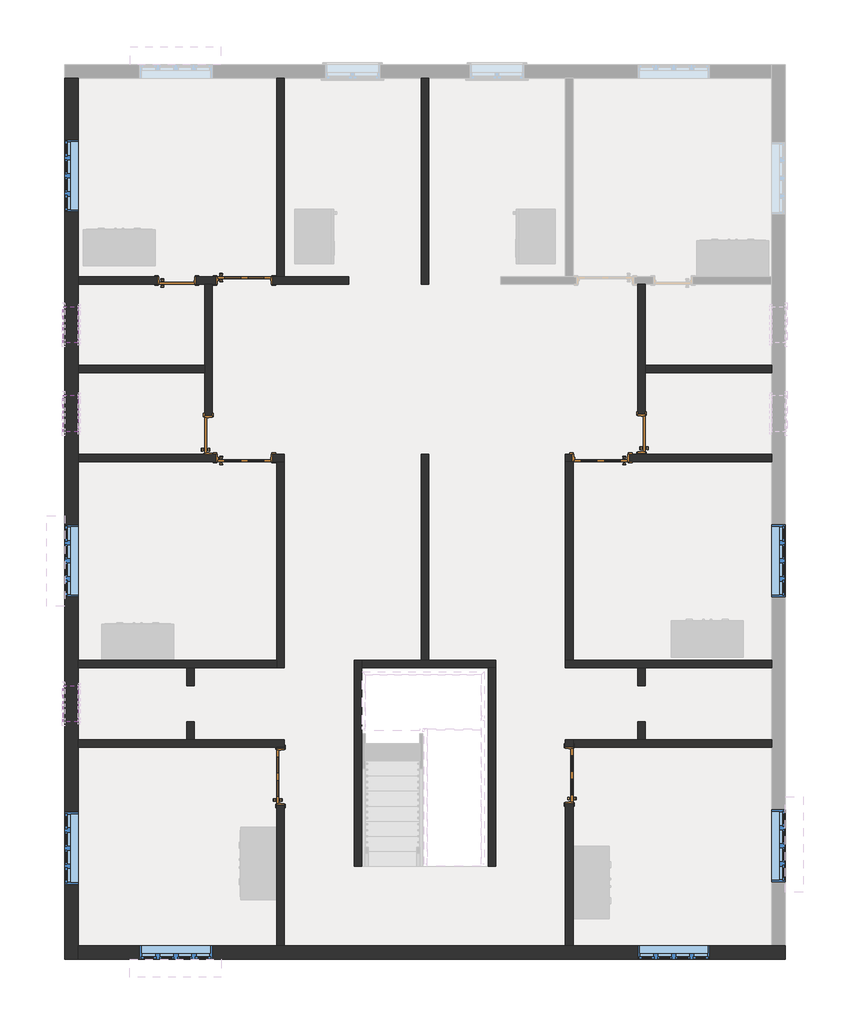
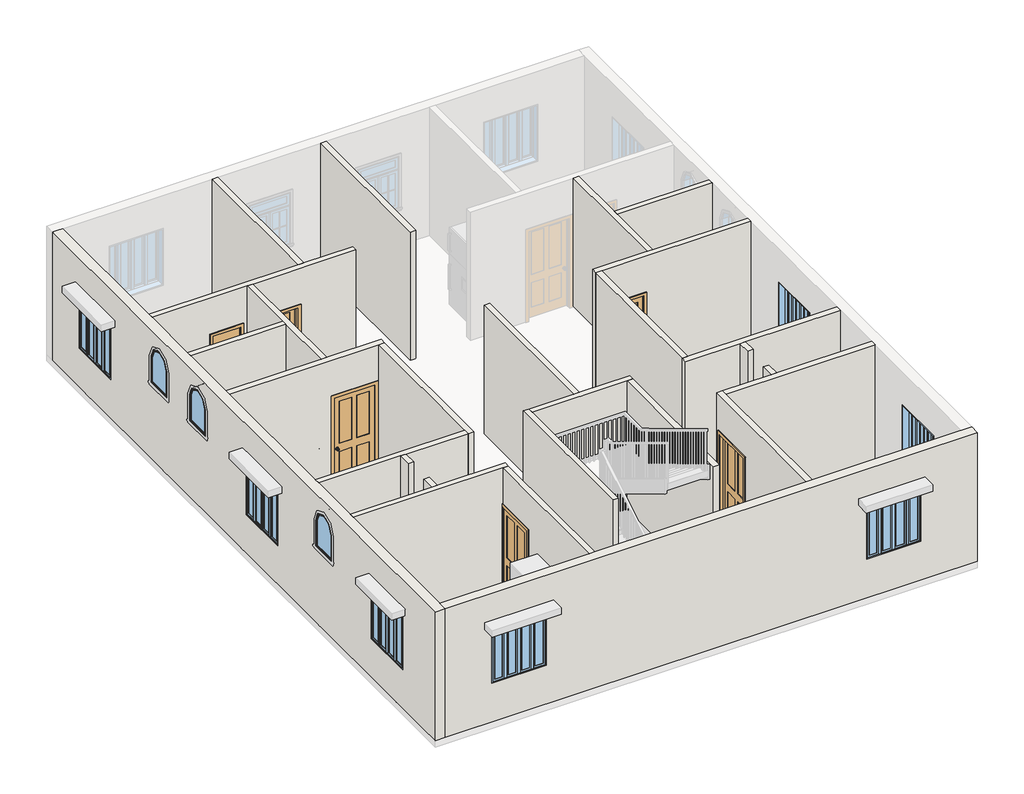
# One storey, part 1 of 4: 27 walls, 10 windows, 8 doors.
"""IFC4 building model written with IfcOpenShell, lengths in millimetres."""

from ifc_helpers import new_model, si_unit, frame, origin, place, context, project, spatial, polyline, circle_curve, outline, extrude, faceted_brep, transform, mapped, element, save
from ifc_brep_helpers import plane_surface, revolved_surface, advanced_brep
from components import door_a823658d, door_68a706ac, door_3f5f64ee, door_428b1ac9, window_casement_multi_sash_horizontal_main_windows_4_x_7_0e27d311, window_casement_multi_sash_horizontal_main_windows_4_x_7_c0e1ebbb, window_2fd4accf

model = new_model("IFC4")

# Units and contexts
model_context = context("Model", 3, world=origin())
ifc_project = project(units=[si_unit("LENGTHUNIT", "METRE", prefix="MILLI")], contexts=[model_context])

# Site, building, storey
site = spatial("IfcSite", under=ifc_project)
building = spatial("IfcBuilding", under=site)
storey = spatial("IfcBuildingStorey", under=building, Elevation=3352.8)

# Doors
placement = place(None, origin())
door_shape = door_a823658d(model_context)
element("IfcDoor", 1, ObjectType="Door-Interior-Single-4_Panel-Wood : 36\" x 84\"", at=placement, inside=storey, context=model_context, shape_type="MappedRepresentation", body=[
    mapped(door_shape, transform((-7097.4021954, -3420.7727897, 3352.8), x_axis=(0.0, 1.0, 0.0), y_axis=(-1.0, 0.0, 0.0), z_axis=(0.0, 0.0, 1.0))),
])
element("IfcDoor", 2, ObjectType="Door-Interior-Single-4_Panel-Wood : 36\" x 84\"", at=placement, inside=storey, context=model_context, shape_type="MappedRepresentation", body=[
    mapped(door_shape, transform((-12586.9771954, 1935.9816069, 3352.8), x_axis=(1.0, 0.0, 0.0), y_axis=(0.0, 1.0, 0.0), z_axis=(0.0, 0.0, 1.0))),
])
door_2_shape = door_68a706ac(model_context)
element("IfcDoor", 3, ObjectType="Door-Interior-Single-4_Panel-Wood : 36\" x 84\"", at=placement, inside=storey, context=model_context, shape_type="MappedRepresentation", body=[
    mapped(door_2_shape, transform((-11980.5521954, -3446.1727897, 3352.8), x_axis=(0.0, 1.0, 0.0), y_axis=(-1.0, 0.0, 0.0), z_axis=(0.0, 0.0, 1.0))),
])
element("IfcDoor", 4, ObjectType="Door-Interior-Single-4_Panel-Wood : 36\" x 84\"", at=placement, inside=storey, context=model_context, shape_type="MappedRepresentation", body=[
    mapped(door_2_shape, transform((-6567.1771954, 1935.9816069, 3352.8), x_axis=(-1.0, 0.0, 0.0), y_axis=(0.0, -1.0, 0.0), z_axis=(0.0, 0.0, 1.0))),
])
element("IfcDoor", 5, ObjectType="Door-Interior-Single-4_Panel-Wood : 36\" x 84\"", at=placement, inside=storey, context=model_context, shape_type="MappedRepresentation", body=[
    mapped(door_2_shape, transform((-12586.9771954, 4939.0022103, 3352.8), x_axis=(1.0, 0.0, 0.0), y_axis=(0.0, 1.0, 0.0), z_axis=(0.0, 0.0, 1.0))),
])
door_3_shape = door_3f5f64ee(model_context)
element("IfcDoor", 6, ObjectType="Door-Interior-Single-Flush_Panel-Wood : 24\" x 84\"", at=placement, inside=storey, context=model_context, shape_type="MappedRepresentation", body=[
    mapped(door_3_shape, transform((-13199.7521954, 2320.1566069, 3352.8), x_axis=(0.0, 1.0, 0.0), y_axis=(-1.0, 0.0, 0.0), z_axis=(0.0, 0.0, 1.0))),
])
door_4_shape = door_428b1ac9(model_context)
element("IfcDoor", 7, ObjectType="Door-Interior-Single-Flush_Panel-Wood : 24\" x 84\"", at=placement, inside=storey, context=model_context, shape_type="MappedRepresentation", body=[
    mapped(door_4_shape, transform((-13729.9771954, 4932.6522103, 3352.8), x_axis=(1.0, 0.0, 0.0), y_axis=(0.0, 1.0, 0.0), z_axis=(0.0, 0.0, 1.0))),
])
element("IfcDoor", 8, ObjectType="Door-Interior-Single-Flush_Panel-Wood : 24\" x 84\"", at=placement, inside=storey, context=model_context, shape_type="MappedRepresentation", body=[
    mapped(door_4_shape, transform((-5878.2021954, 2345.5566069, 3352.8), x_axis=(0.0, 1.0, 0.0), y_axis=(-1.0, 0.0, 0.0), z_axis=(0.0, 0.0, 1.0))),
])

# Walls
element("IfcWall", 9, ObjectType="INNER WALL 5\"", at=placement, inside=storey, context=model_context, shape_type="Brep", body=[
    faceted_brep([(-10821.6771954, 4872.3272103, 3352.8), (-10821.6771954, 4872.3272103, 6400.8), (-13133.0771954, 4872.3272103, 6400.8), (-13260.0771954, 4872.3272103, 6400.8), (-15395.2646954, 4872.3272103, 6400.8), (-15395.2646954, 4872.3272103, 3352.8), (-14060.1771954, 4872.3272103, 3352.8), (-14060.1771954, 4872.3272103, 5511.8), (-13399.7771954, 4872.3272103, 5511.8), (-13399.7771954, 4872.3272103, 3352.8), (-13260.0771954, 4872.3272103, 3352.8), (-13133.0771954, 4872.3272103, 3352.8), (-13069.5771954, 4872.3272103, 3352.8), (-13069.5771954, 4872.3272103, 5511.8), (-12104.3771954, 4872.3272103, 5511.8), (-12104.3771954, 4872.3272103, 3352.8), (-10821.6771954, 4999.3272103, 6400.8), (-10821.6771954, 4999.3272103, 3352.8), (-11913.8771954, 4999.3272103, 3352.8), (-12040.8771954, 4999.3272103, 3352.8), (-12104.3771954, 4999.3272103, 3352.8), (-12104.3771954, 4999.3272103, 5511.8), (-13069.5771954, 4999.3272103, 5511.8), (-13069.5771954, 4999.3272103, 3352.8), (-13399.7771954, 4999.3272103, 3352.8), (-13399.7771954, 4999.3272103, 5511.8), (-14060.1771954, 4999.3272103, 5511.8), (-14060.1771954, 4999.3272103, 3352.8), (-15395.2646954, 4999.3272103, 3352.8), (-15395.2646954, 4999.3272103, 6400.8), (-12040.8771954, 4999.3272103, 6400.8), (-11913.8771954, 4999.3272103, 6400.8)], [[[0, 1, 2, 3, 4, 5, 6, 7, 8, 9, 10, 11, 12, 13, 14, 15]], [[16, 17, 18, 19, 20, 21, 22, 23, 24, 25, 26, 27, 28, 29, 30, 31]], [[17, 0, 15, 20, 19, 18]], [[5, 28, 27, 6]], [[23, 12, 11, 10, 9, 24]], [[1, 0, 17, 16]], [[4, 3, 2, 1, 16, 31, 30, 29]], [[5, 4, 29, 28]], [[14, 21, 20, 15]], [[21, 14, 13, 22]], [[22, 13, 12, 23]], [[8, 25, 24, 9]], [[25, 8, 7, 26]], [[26, 7, 6, 27]]]),
])
element("IfcWall", 10, ObjectType="INNER WALL 5\"", at=placement, inside=storey, context=model_context, shape_type="SweptSolid", body=[
    extrude(outline(polyline([(-12040.8771954, 4999.3272103), (-12040.8771954, 8352.1272103), (-11913.8771954, 8352.1272103), (-11913.8771954, 4999.3272103), (-12040.8771954, 4999.3272103)])), frame((0.0, 0.0, 3352.8), z_axis=(0.0, 0.0, 1.0), x_axis=(1.0, 0.0, 0.0)), (0.0, 0.0, 1.0), 3048.0),
])
element("IfcWall", 11, ObjectType="INNER WALL 5\"", at=placement, inside=storey, context=model_context, shape_type="SweptSolid", body=[
    extrude(outline(polyline([(-9602.4771954, 4872.3272103), (-9602.4771954, 8352.1272103), (-9475.4771954, 8352.1272103), (-9475.4771954, 4872.3272103), (-9602.4771954, 4872.3272103)])), frame((0.0, 0.0, 3352.8), z_axis=(0.0, 0.0, 1.0), x_axis=(1.0, 0.0, 0.0)), (0.0, 0.0, 1.0), 3048.0),
])
element("IfcWall", 12, ObjectType="INNER WALL 5\"", at=placement, inside=storey, context=model_context, shape_type="SweptSolid", body=[
    extrude(outline(polyline([(-13260.0771954, 3373.7272103), (-15395.2646954, 3373.7272103), (-15395.2646954, 3500.7272103), (-13260.0771954, 3500.7272103), (-13260.0771954, 3373.7272103)])), frame((0.0, 0.0, 3352.8), z_axis=(0.0, 0.0, 1.0), x_axis=(1.0, 0.0, 0.0)), (0.0, 0.0, 1.0), 3048.0),
])
element("IfcWall", 13, ObjectType="INNER WALL 5\"", at=placement, inside=storey, context=model_context, shape_type="Brep", body=[
    faceted_brep([(-13260.0771954, 2002.6566069, 6400.8), (-13260.0771954, 3373.7272103, 6400.8), (-13260.0771954, 3500.7272103, 6400.8), (-13260.0771954, 4872.3272103, 6400.8), (-13260.0771954, 4872.3272103, 3352.8), (-13260.0771954, 3500.7272103, 3352.8), (-13260.0771954, 3373.7272103, 3352.8), (-13260.0771954, 2650.3566069, 3352.8), (-13260.0771954, 2650.3566069, 5511.8), (-13260.0771954, 2002.6566069, 5511.8), (-13133.0771954, 4872.3272103, 6400.8), (-13133.0771954, 2002.6566069, 6400.8), (-13133.0771954, 2002.6566069, 5511.8), (-13133.0771954, 2650.3566069, 5511.8), (-13133.0771954, 2650.3566069, 3352.8), (-13133.0771954, 4872.3272103, 3352.8)], [[[0, 1, 2, 3, 4, 5, 6, 7, 8, 9]], [[10, 11, 12, 13, 14, 15]], [[4, 15, 14, 7, 6, 5]], [[3, 2, 1, 0, 11, 10]], [[4, 3, 10, 15]], [[11, 0, 9, 12]], [[13, 8, 7, 14]], [[8, 13, 12, 9]]]),
])
element("IfcWall", 14, ObjectType="INNER WALL 5\"", at=placement, inside=storey, context=model_context, shape_type="Brep", body=[
    faceted_brep([(-11913.8771954, 1875.6566069, 6400.8), (-12040.8771954, 1875.6566069, 6400.8), (-15395.2646954, 1875.6566069, 6400.8), (-15395.2646954, 1875.6566069, 3352.8), (-13069.5771954, 1875.6566069, 3352.8), (-13069.5771954, 1875.6566069, 5511.8), (-12104.3771954, 1875.6566069, 5511.8), (-12104.3771954, 1875.6566069, 3352.8), (-12040.8771954, 1875.6566069, 3352.8), (-11913.8771954, 1875.6566069, 3352.8), (-15395.2646954, 2002.6566069, 6400.8), (-13260.0771954, 2002.6566069, 6400.8), (-13133.0771954, 2002.6566069, 6400.8), (-11913.8771954, 2002.6566069, 6400.8), (-11913.8771954, 2002.6566069, 3352.8), (-12104.3771954, 2002.6566069, 3352.8), (-12104.3771954, 2002.6566069, 5511.8), (-13069.5771954, 2002.6566069, 5511.8), (-13069.5771954, 2002.6566069, 3352.8), (-13133.0771954, 2002.6566069, 3352.8), (-13133.0771954, 2002.6566069, 5511.8), (-13260.0771954, 2002.6566069, 5511.8), (-13260.0771954, 2002.6566069, 3352.8), (-15395.2646954, 2002.6566069, 3352.8), (-13260.0771954, 1989.9566069, 3352.8), (-13133.0771954, 1989.9566069, 3352.8), (-13133.0771954, 1989.9566069, 5511.8), (-13260.0771954, 1989.9566069, 5511.8)], [[[0, 1, 2, 3, 4, 5, 6, 7, 8, 9]], [[10, 11, 12, 13, 14, 15, 16, 17, 18, 19, 20, 21, 22, 23]], [[3, 23, 22, 24, 25, 19, 18, 4]], [[14, 9, 8, 7, 15]], [[2, 1, 0, 13, 12, 11, 10]], [[3, 2, 10, 23]], [[0, 9, 14, 13]], [[6, 16, 15, 7]], [[16, 6, 5, 17]], [[17, 5, 4, 18]], [[25, 26, 20, 19]], [[27, 24, 22, 21]], [[26, 27, 21, 20]], [[26, 25, 24, 27]]]),
])
element("IfcWall", 15, ObjectType="INNER WALL 5\"", at=placement, inside=storey, context=model_context, shape_type="SweptSolid", body=[
    extrude(outline(polyline([(-9602.4771954, -1477.6727897), (-9602.4771954, 2002.6566069), (-9475.4771954, 2002.6566069), (-9475.4771954, -1477.6727897), (-9602.4771954, -1477.6727897)])), frame((0.0, 0.0, 3352.8), z_axis=(0.0, 0.0, 1.0), x_axis=(1.0, 0.0, 0.0)), (0.0, 0.0, 1.0), 3048.0),
])
element("IfcWall", 16, ObjectType="INNER WALL 5\"", at=placement, inside=storey, context=model_context, shape_type="Brep", body=[
    faceted_brep([(-5944.8771954, 2002.6566069, 6400.8), (-5944.8771954, 4872.3272103, 6400.8), (-5944.8771954, 4872.3272103, 3352.8), (-5944.8771954, 2675.7566069, 3352.8), (-5944.8771954, 2675.7566069, 5511.8), (-5944.8771954, 2015.3566069, 5511.8), (-5944.8771954, 2015.3566069, 3352.8), (-5944.8771954, 2002.6566069, 3352.8), (-5817.8771954, 4872.3272103, 6400.8), (-5817.8771954, 3500.7272103, 6400.8), (-5817.8771954, 3373.7272103, 6400.8), (-5817.8771954, 2002.6566069, 6400.8), (-5817.8771954, 2002.6566069, 3352.8), (-5817.8771954, 2015.3566069, 3352.8), (-5817.8771954, 2015.3566069, 5511.8), (-5817.8771954, 2675.7566069, 5511.8), (-5817.8771954, 2675.7566069, 3352.8), (-5817.8771954, 3373.7272103, 3352.8), (-5817.8771954, 3500.7272103, 3352.8), (-5817.8771954, 4872.3272103, 3352.8)], [[[0, 1, 2, 3, 4, 5, 6, 7]], [[8, 9, 10, 11, 12, 13, 14, 15, 16, 17, 18, 19]], [[2, 19, 18, 17, 16, 3]], [[12, 7, 6, 13]], [[1, 0, 11, 10, 9, 8]], [[2, 1, 8, 19]], [[0, 7, 12, 11]], [[15, 4, 3, 16]], [[4, 15, 14, 5]], [[5, 14, 13, 6]]]),
])
element("IfcWall", 17, ObjectType="INNER WALL 5\"", at=placement, inside=storey, context=model_context, shape_type="SweptSolid", body=[
    extrude(outline(polyline([(-3684.2771954, 3373.7272103), (-5817.8771954, 3373.7272103), (-5817.8771954, 3500.7272103), (-3684.2771954, 3500.7272103), (-3684.2771954, 3373.7272103)])), frame((0.0, 0.0, 3352.8), z_axis=(0.0, 0.0, 1.0), x_axis=(1.0, 0.0, 0.0)), (0.0, 0.0, 1.0), 3048.0),
])
element("IfcWall", 18, ObjectType="INNER WALL 5\"", at=placement, inside=storey, context=model_context, shape_type="Brep", body=[
    faceted_brep([(-7164.0771954, 2002.6566069, 6400.8), (-5944.8771954, 2002.6566069, 6400.8), (-5817.8771954, 2002.6566069, 6400.8), (-3684.2771954, 2002.6566069, 6400.8), (-3684.2771954, 2002.6566069, 3352.8), (-5817.8771954, 2002.6566069, 3352.8), (-5944.8771954, 2002.6566069, 3352.8), (-6084.5771954, 2002.6566069, 3352.8), (-6084.5771954, 2002.6566069, 5511.8), (-7049.7771954, 2002.6566069, 5511.8), (-7049.7771954, 2002.6566069, 3352.8), (-7164.0771954, 2002.6566069, 3352.8), (-3684.2771954, 1875.6566069, 6400.8), (-7037.0771954, 1875.6566069, 6400.8), (-7164.0771954, 1875.6566069, 6400.8), (-7164.0771954, 1875.6566069, 3352.8), (-7049.7771954, 1875.6566069, 3352.8), (-7049.7771954, 1875.6566069, 5511.8), (-6084.5771954, 1875.6566069, 5511.8), (-6084.5771954, 1875.6566069, 3352.8), (-3684.2771954, 1875.6566069, 3352.8)], [[[0, 1, 2, 3, 4, 5, 6, 7, 8, 9, 10, 11]], [[12, 13, 14, 15, 16, 17, 18, 19, 20]], [[4, 20, 19, 7, 6, 5]], [[15, 11, 10, 16]], [[3, 2, 1, 0, 14, 13, 12]], [[4, 3, 12, 20]], [[0, 11, 15, 14]], [[9, 17, 16, 10]], [[17, 9, 8, 18]], [[18, 8, 7, 19]]]),
])
element("IfcWall", 19, ObjectType="INNER WALL 5\"", at=placement, inside=storey, context=model_context, shape_type="Brep", body=[
    faceted_brep([(-12040.8771954, 1875.6566069, 3352.8), (-12040.8771954, -1477.6727897, 3352.8), (-12040.8771954, -1604.6727897, 3352.8), (-12040.8771954, -1604.6727897, 6400.8), (-12040.8771954, -1477.6727897, 6400.8), (-12040.8771954, 1875.6566069, 6400.8), (-11913.8771954, 1875.6566069, 3352.8), (-11913.8771954, 1875.6566069, 6400.8), (-11913.8771954, -1604.6727897, 6400.8), (-11913.8771954, -1604.6727897, 3352.8)], [[[0, 1, 2, 3, 4, 5]], [[6, 7, 8, 9]], [[2, 1, 0, 6, 9]], [[5, 4, 3, 8, 7]], [[0, 5, 7, 6]], [[3, 2, 9, 8]]]),
])
element("IfcWall", 20, ObjectType="INNER WALL 5\"", at=placement, inside=storey, context=model_context, shape_type="Brep", body=[
    faceted_brep([(-12040.8771954, -1477.6727897, 3352.8), (-15395.2646954, -1477.6727897, 3352.8), (-15395.2646954, -1477.6727897, 6400.8), (-12040.8771954, -1477.6727897, 6400.8), (-12040.8771954, -1604.6727897, 3352.8), (-12040.8771954, -1604.6727897, 6400.8), (-13437.8771954, -1604.6727897, 6400.8), (-13564.8771954, -1604.6727897, 6400.8), (-15395.2646954, -1604.6727897, 6400.8), (-15395.2646954, -1604.6727897, 3352.8), (-13564.8771954, -1604.6727897, 3352.8), (-13437.8771954, -1604.6727897, 3352.8)], [[[0, 1, 2, 3]], [[4, 5, 6, 7, 8, 9, 10, 11]], [[1, 0, 4, 11, 10, 9]], [[3, 2, 8, 7, 6, 5]], [[0, 3, 5, 4]], [[2, 1, 9, 8]]]),
])
element("IfcWall", 21, ObjectType="INNER WALL 5\"", at=placement, inside=storey, context=model_context, shape_type="Brep", body=[
    faceted_brep([(-15395.2646954, -2950.8727897, 3352.8), (-12040.8771954, -2950.8727897, 3352.8), (-11913.8771954, -2950.8727897, 3352.8), (-11913.8771954, -2950.8727897, 6400.8), (-12040.8771954, -2950.8727897, 6400.8), (-15395.2646954, -2950.8727897, 6400.8), (-15395.2646954, -2823.8727897, 3352.8), (-15395.2646954, -2823.8727897, 6400.8), (-13564.8771954, -2823.8727897, 6400.8), (-13437.8771954, -2823.8727897, 6400.8), (-11913.8771954, -2823.8727897, 6400.8), (-11913.8771954, -2823.8727897, 3352.8), (-13437.8771954, -2823.8727897, 3352.8), (-13564.8771954, -2823.8727897, 3352.8)], [[[0, 1, 2, 3, 4, 5]], [[6, 7, 8, 9, 10, 11, 12, 13]], [[2, 1, 0, 6, 13, 12, 11]], [[5, 4, 3, 10, 9, 8, 7]], [[0, 5, 7, 6]], [[3, 2, 11, 10]]]),
])
element("IfcWall", 22, ObjectType="INNER WALL 5\"", at=placement, inside=storey, context=model_context, shape_type="SweptSolid", body=[
    extrude(outline(polyline([(-6303.6727897, 6400.8), (-2950.8727897, 6400.8), (-2950.8727897, 3352.8), (-2963.5727897, 3352.8), (-2963.5727897, 5511.8), (-3928.7727897, 5511.8), (-3928.7727897, 3352.8), (-6303.6727897, 3352.8), (-6303.6727897, 6400.8)])), frame((-12040.8771954, 0.0, 0.0), z_axis=(1.0, 0.0, 0.0), x_axis=(0.0, 1.0, 0.0)), (0.0, 0.0, 1.0), 127.0),
])
element("IfcWall", 23, ObjectType="INNER WALL 5\"", at=placement, inside=storey, context=model_context, shape_type="Brep", body=[
    faceted_brep([(-7037.0771954, -2823.8727897, 6400.8), (-7037.0771954, -2950.8727897, 6400.8), (-7037.0771954, -6303.6727897, 6400.8), (-7037.0771954, -6303.6727897, 3352.8), (-7037.0771954, -3903.3727897, 3352.8), (-7037.0771954, -3903.3727897, 5511.8), (-7037.0771954, -2938.1727897, 5511.8), (-7037.0771954, -2938.1727897, 3352.8), (-7037.0771954, -2823.8727897, 3352.8), (-7164.0771954, -6303.6727897, 6400.8), (-7164.0771954, -2823.8727897, 6400.8), (-7164.0771954, -2823.8727897, 3352.8), (-7164.0771954, -2938.1727897, 3352.8), (-7164.0771954, -2938.1727897, 5511.8), (-7164.0771954, -3903.3727897, 5511.8), (-7164.0771954, -3903.3727897, 3352.8), (-7164.0771954, -6303.6727897, 3352.8)], [[[0, 1, 2, 3, 4, 5, 6, 7, 8]], [[9, 10, 11, 12, 13, 14, 15, 16]], [[3, 16, 15, 4]], [[11, 8, 7, 12]], [[2, 1, 0, 10, 9]], [[3, 2, 9, 16]], [[0, 8, 11, 10]], [[6, 13, 12, 7]], [[13, 6, 5, 14]], [[14, 5, 4, 15]]]),
])
element("IfcWall", 24, ObjectType="INNER WALL 5\"", at=placement, inside=storey, context=model_context, shape_type="Brep", body=[
    faceted_brep([(-3684.2771954, -2823.8727897, 3352.8), (-5817.8771954, -2823.8727897, 3352.8), (-5944.8771954, -2823.8727897, 3352.8), (-7037.0771954, -2823.8727897, 3352.8), (-7037.0771954, -2823.8727897, 6400.8), (-5944.8771954, -2823.8727897, 6400.8), (-5817.8771954, -2823.8727897, 6400.8), (-3684.2771954, -2823.8727897, 6400.8), (-3684.2771954, -2950.8727897, 3352.8), (-3684.2771954, -2950.8727897, 6400.8), (-7037.0771954, -2950.8727897, 6400.8), (-7037.0771954, -2950.8727897, 3352.8)], [[[0, 1, 2, 3, 4, 5, 6, 7]], [[8, 9, 10, 11]], [[3, 2, 1, 0, 8, 11]], [[7, 6, 5, 4, 10, 9]], [[4, 3, 11, 10]], [[0, 7, 9, 8]]]),
])
element("IfcWall", 25, ObjectType="INNER WALL 5\"", at=placement, inside=storey, context=model_context, shape_type="Brep", body=[
    faceted_brep([(-3684.2771954, -1477.6727897, 3352.8), (-7037.0771954, -1477.6727897, 3352.8), (-7164.0771954, -1477.6727897, 3352.8), (-7164.0771954, -1477.6727897, 6400.8), (-7037.0771954, -1477.6727897, 6400.8), (-3684.2771954, -1477.6727897, 6400.8), (-3684.2771954, -1604.6727897, 3352.8), (-3684.2771954, -1604.6727897, 6400.8), (-5817.8771954, -1604.6727897, 6400.8), (-5944.8771954, -1604.6727897, 6400.8), (-7164.0771954, -1604.6727897, 6400.8), (-7164.0771954, -1604.6727897, 3352.8), (-5944.8771954, -1604.6727897, 3352.8), (-5817.8771954, -1604.6727897, 3352.8)], [[[0, 1, 2, 3, 4, 5]], [[6, 7, 8, 9, 10, 11, 12, 13]], [[2, 1, 0, 6, 13, 12, 11]], [[5, 4, 3, 10, 9, 8, 7]], [[0, 5, 7, 6]], [[3, 2, 11, 10]]]),
])
element("IfcWall", 26, ObjectType="INNER WALL 5\"", at=placement, inside=storey, context=model_context, shape_type="SweptSolid", body=[
    extrude(outline(polyline([(-7037.0771954, 1875.6566069), (-7037.0771954, -1477.6727897), (-7164.0771954, -1477.6727897), (-7164.0771954, 1875.6566069), (-7037.0771954, 1875.6566069)])), frame((0.0, 0.0, 3352.8), z_axis=(0.0, 0.0, 1.0), x_axis=(1.0, 0.0, 0.0)), (0.0, 0.0, 1.0), 3048.0),
])
element("IfcWall", 27, ObjectType="INNER WALL 5\"", at=placement, inside=storey, context=model_context, shape_type="SweptSolid", body=[
    extrude(outline(polyline([(-13564.8771954, -1909.4727897), (-13564.8771954, -1604.6727897), (-13437.8771954, -1604.6727897), (-13437.8771954, -1909.4727897), (-13564.8771954, -1909.4727897)])), frame((0.0, 0.0, 3352.8), z_axis=(0.0, 0.0, 1.0), x_axis=(1.0, 0.0, 0.0)), (0.0, 0.0, 1.0), 3048.0),
])
element("IfcWall", 28, ObjectType="INNER WALL 5\"", at=placement, inside=storey, context=model_context, shape_type="SweptSolid", body=[
    extrude(outline(polyline([(-13437.8771954, -2519.0727897), (-13437.8771954, -2823.8727897), (-13564.8771954, -2823.8727897), (-13564.8771954, -2519.0727897), (-13437.8771954, -2519.0727897)])), frame((0.0, 0.0, 3352.8), z_axis=(0.0, 0.0, 1.0), x_axis=(1.0, 0.0, 0.0)), (0.0, 0.0, 1.0), 3048.0),
])
element("IfcWall", 29, ObjectType="INNER WALL 5\"", at=placement, inside=storey, context=model_context, shape_type="SweptSolid", body=[
    extrude(outline(polyline([(-5817.8771954, -2519.0727897), (-5817.8771954, -2823.8727897), (-5944.8771954, -2823.8727897), (-5944.8771954, -2519.0727897), (-5817.8771954, -2519.0727897)])), frame((0.0, 0.0, 3352.8), z_axis=(0.0, 0.0, 1.0), x_axis=(1.0, 0.0, 0.0)), (0.0, 0.0, 1.0), 3048.0),
])
element("IfcWall", 30, ObjectType="INNER WALL 5\"", at=placement, inside=storey, context=model_context, shape_type="SweptSolid", body=[
    extrude(outline(polyline([(-5944.8771954, -1909.4727897), (-5944.8771954, -1604.6727897), (-5817.8771954, -1604.6727897), (-5817.8771954, -1909.4727897), (-5944.8771954, -1909.4727897)])), frame((0.0, 0.0, 3352.8), z_axis=(0.0, 0.0, 1.0), x_axis=(1.0, 0.0, 0.0)), (0.0, 0.0, 1.0), 3048.0),
])
element("IfcWall", 31, ObjectType="INNER WALL 5\"", at=placement, inside=storey, context=model_context, shape_type="Brep", body=[
    faceted_brep([(-10605.7771954, -4957.4727897, 3352.8), (-10605.7771954, -1604.6727897, 3352.8), (-10605.7771954, -1477.6727897, 3352.8), (-10605.7771954, -1477.6727897, 6400.8), (-10605.7771954, -1604.6727897, 6400.8), (-10605.7771954, -4957.4727897, 6400.8), (-10732.7771954, -4957.4727897, 3352.8), (-10732.7771954, -4957.4727897, 6400.8), (-10732.7771954, -1477.6727897, 6400.8), (-10732.7771954, -1477.6727897, 3352.8)], [[[0, 1, 2, 3, 4, 5]], [[6, 7, 8, 9]], [[2, 1, 0, 6, 9]], [[5, 4, 3, 8, 7]], [[0, 5, 7, 6]], [[3, 2, 9, 8]]]),
])
element("IfcWall", 32, ObjectType="INNER WALL 5\"", at=placement, inside=storey, context=model_context, shape_type="Brep", body=[
    faceted_brep([(-10605.7771954, -1604.6727897, 3352.8), (-8472.1771954, -1604.6727897, 3352.8), (-8345.1771954, -1604.6727897, 3352.8), (-8345.1771954, -1604.6727897, 6400.8), (-8472.1771954, -1604.6727897, 6400.8), (-10605.7771954, -1604.6727897, 6400.8), (-10605.7771954, -1477.6727897, 3352.8), (-10605.7771954, -1477.6727897, 6400.8), (-9602.4771954, -1477.6727897, 6400.8), (-9475.4771954, -1477.6727897, 6400.8), (-8345.1771954, -1477.6727897, 6400.8), (-8345.1771954, -1477.6727897, 3352.8), (-9475.4771954, -1477.6727897, 3352.8), (-9602.4771954, -1477.6727897, 3352.8)], [[[0, 1, 2, 3, 4, 5]], [[6, 7, 8, 9, 10, 11, 12, 13]], [[2, 1, 0, 6, 13, 12, 11]], [[5, 4, 3, 10, 9, 8, 7]], [[0, 5, 7, 6]], [[3, 2, 11, 10]]]),
])
element("IfcWall", 33, ObjectType="INNER WALL 5\"", at=placement, inside=storey, context=model_context, shape_type="SweptSolid", body=[
    extrude(outline(polyline([(-8472.1771954, -4957.4727897), (-8472.1771954, -1604.6727897), (-8345.1771954, -1604.6727897), (-8345.1771954, -4957.4727897), (-8472.1771954, -4957.4727897)])), frame((0.0, 0.0, 3352.8), z_axis=(0.0, 0.0, 1.0), x_axis=(1.0, 0.0, 0.0)), (0.0, 0.0, 1.0), 3048.0),
])
element("IfcWall", 34, ObjectType="OUTER WALL 9\"", at=placement, inside=storey, context=model_context, shape_type="AdvancedBrep", body=[
    advanced_brep(
    [(-15395.2646954, -6532.2727897, 3352.8), (-15395.2646954, -6303.6727897, 3352.8), (-15395.2646954, -2950.8727897, 3352.8), (-15395.2646954, -2823.8727897, 3352.8), (-15395.2646954, -1604.6727897, 3352.8), (-15395.2646954, -1477.6727897, 3352.8), (-15395.2646954, 1875.6566069, 3352.8), (-15395.2646954, 2002.6566069, 3352.8), (-15395.2646954, 3373.7272103, 3352.8), (-15395.2646954, 3500.7272103, 3352.8), (-15395.2646954, 4872.3272103, 3352.8), (-15395.2646954, 4999.3272103, 3352.8), (-15395.2646954, 8352.1272103, 3352.8), (-15395.2646954, 8352.1272103, 6400.8), (-15395.2646954, 4999.3272103, 6400.8), (-15395.2646954, 4872.3272103, 6400.8), (-15395.2646954, 3500.7272103, 6400.8), (-15395.2646954, 3373.7272103, 6400.8), (-15395.2646954, 2002.6566069, 6400.8), (-15395.2646954, 1875.6566069, 6400.8), (-15395.2646954, -1477.6727897, 6400.8), (-15395.2646954, -1604.6727897, 6400.8), (-15395.2646954, -2823.8727897, 6400.8), (-15395.2646954, -2950.8727897, 6400.8), (-15395.2646954, -6303.6727897, 6400.8), (-15395.2646954, -6532.2727897, 6400.8), (-15395.2646954, -4043.0727897, 5613.4), (-15395.2646954, -4043.0727897, 4267.2), (-15395.2646954, -5262.2727897, 4267.2), (-15395.2646954, -5262.2727897, 5613.4), (-15395.2646954, 808.5919086, 5613.4), (-15395.2646954, 808.5919086, 4267.2), (-15395.2646954, -410.6080914, 4267.2), (-15395.2646954, -410.6080914, 5613.4), (-15395.2646954, 7310.7272103, 5613.4), (-15395.2646954, 7310.7272103, 4267.2), (-15395.2646954, 6091.5272103, 4267.2), (-15395.2646954, 6091.5272103, 5613.4), (-15395.2646954, -2519.0727897, 5181.6), (-15395.2646954, -2519.0727897, 5791.2), (-15395.2646954, -1909.4727897, 5791.2), (-15395.2646954, -1909.4727897, 5181.6), (-15395.2646954, 2383.3919086, 5181.6), (-15395.2646954, 2383.3919086, 5791.2), (-15395.2646954, 2992.9919086, 5791.2), (-15395.2646954, 2992.9919086, 5181.6), (-15395.2646954, 3881.7272103, 5181.6), (-15395.2646954, 3881.7272103, 5791.2), (-15395.2646954, 4491.3272103, 5791.2), (-15395.2646954, 4491.3272103, 5181.6), (-15623.8646954, -6532.2727897, 3352.8), (-15623.8646954, -6532.2727897, 6400.8), (-15623.8646954, 8352.1272103, 6400.8), (-15623.8646954, 8352.1272103, 3352.8), (-15623.8646954, -4043.0727897, 5613.4), (-15623.8646954, -5262.2727897, 5613.4), (-15623.8646954, -5262.2727897, 4267.2), (-15623.8646954, -4043.0727897, 4267.2), (-15623.8646954, 808.5919086, 5613.4), (-15623.8646954, -410.6080914, 5613.4), (-15623.8646954, -410.6080914, 4267.2), (-15623.8646954, 808.5919086, 4267.2), (-15623.8646954, 7310.7272103, 5613.4), (-15623.8646954, 6091.5272103, 5613.4), (-15623.8646954, 6091.5272103, 4267.2), (-15623.8646954, 7310.7272103, 4267.2), (-15623.8646954, -2519.0727897, 5181.6), (-15623.8646954, -1909.4727897, 5181.6), (-15623.8646954, -1909.4727897, 5791.2), (-15623.8646954, -2519.0727897, 5791.2), (-15623.8646954, 2383.3919086, 5181.6), (-15623.8646954, 2992.9919086, 5181.6), (-15623.8646954, 2992.9919086, 5791.2), (-15623.8646954, 2383.3919086, 5791.2), (-15623.8646954, 3881.7272103, 5181.6), (-15623.8646954, 4491.3272103, 5181.6), (-15623.8646954, 4491.3272103, 5791.2), (-15623.8646954, 3881.7272103, 5791.2)],
    [
        (0, 1),
        (1, 2),
        (2, 3),
        (3, 4),
        (4, 5),
        (5, 6),
        (6, 7),
        (7, 8),
        (8, 9),
        (9, 10),
        (10, 11),
        (11, 12),
        (12, 13),
        (13, 14),
        (14, 15),
        (15, 16),
        (16, 17),
        (17, 18),
        (18, 19),
        (19, 20),
        (20, 21),
        (21, 22),
        (22, 23),
        (23, 24),
        (24, 25),
        (25, 0),
        (26, 27),
        (27, 28),
        (28, 29),
        (29, 26),
        (30, 31),
        (31, 32),
        (32, 33),
        (33, 30),
        (34, 35),
        (35, 36),
        (36, 37),
        (37, 34),
        (38, 39),
        (39, 40, circle_curve(frame((-15395.2646954, -2214.2727897, 5791.2), z_axis=(-1.0, 0.0, 0.0), x_axis=(0.0, 1.0, 0.0)), 304.8)),
        (40, 41),
        (41, 38),
        (42, 43),
        (43, 44, circle_curve(frame((-15395.2646954, 2688.1919086, 5791.2), z_axis=(-1.0, 0.0, 0.0), x_axis=(0.0, 1.0, 0.0)), 304.8)),
        (44, 45),
        (45, 42),
        (46, 47),
        (47, 48, circle_curve(frame((-15395.2646954, 4186.5272103, 5791.2), z_axis=(-1.0, 0.0, 0.0), x_axis=(0.0, 1.0, 0.0)), 304.8)),
        (48, 49),
        (49, 46),
        (50, 51),
        (51, 52),
        (52, 53),
        (53, 50),
        (54, 55),
        (55, 56),
        (56, 57),
        (57, 54),
        (58, 59),
        (59, 60),
        (60, 61),
        (61, 58),
        (62, 63),
        (63, 64),
        (64, 65),
        (65, 62),
        (66, 67),
        (67, 68),
        (68, 69, circle_curve(frame((-15623.8646954, -2214.2727897, 5791.2), z_axis=(1.0, 0.0, 0.0), x_axis=(0.0, 1.0, 0.0)), 304.8)),
        (69, 66),
        (70, 71),
        (71, 72),
        (72, 73, circle_curve(frame((-15623.8646954, 2688.1919086, 5791.2), z_axis=(1.0, 0.0, 0.0), x_axis=(0.0, 1.0, 0.0)), 304.8)),
        (73, 70),
        (74, 75),
        (75, 76),
        (76, 77, circle_curve(frame((-15623.8646954, 4186.5272103, 5791.2), z_axis=(1.0, 0.0, 0.0), x_axis=(0.0, 1.0, 0.0)), 304.8)),
        (77, 74),
        (0, 50),
        (53, 12),
        (13, 52),
        (51, 25),
        (26, 54),
        (57, 27),
        (56, 28),
        (55, 29),
        (30, 58),
        (61, 31),
        (60, 32),
        (59, 33),
        (34, 62),
        (65, 35),
        (64, 36),
        (63, 37),
        (66, 38),
        (41, 67),
        (40, 68),
        (39, 69),
        (70, 42),
        (45, 71),
        (44, 72),
        (43, 73),
        (74, 46),
        (49, 75),
        (48, 76),
        (47, 77),
    ],
    [
        plane_surface(frame((-15395.2646954, 7399.6272103, 3352.8), z_axis=(1.0, 0.0, 0.0), x_axis=(0.0, 1.0, 0.0))),
        plane_surface(frame((-15623.8646954, 7399.6272103, 3352.8), z_axis=(-1.0, 0.0, 0.0), x_axis=(0.0, -1.0, 0.0))),
        plane_surface(frame((-15395.2646954, -6417.9727897, 3352.8), z_axis=(0.0, 0.0, -1.0), x_axis=(-1.0, 0.0, 0.0))),
        plane_surface(frame((-15395.2646954, 8466.4272103, 6400.8), z_axis=(0.0, 0.0, 1.0), x_axis=(-1.0, 0.0, 0.0))),
        plane_surface(frame((-3569.9771954, -6532.2727897, 3352.8), z_axis=(0.0, -1.0, 0.0), x_axis=(1.0, 0.0, 0.0))),
        plane_surface(frame((-15509.5646954, 8352.1272103, 3352.8), z_axis=(0.0, 1.0, 0.0), x_axis=(1.0, 0.0, 0.0))),
        plane_surface(frame((-15395.2646954, -4043.0727897, 5613.4), z_axis=(0.0, -1.0, 0.0), x_axis=(-1.0, 0.0, 0.0))),
        plane_surface(frame((-15395.2646954, -4043.0727897, 4267.2), z_axis=(0.0, 0.0, 1.0), x_axis=(-1.0, 0.0, 0.0))),
        plane_surface(frame((-15395.2646954, -5262.2727897, 4267.2), z_axis=(0.0, 1.0, 0.0), x_axis=(-1.0, 0.0, 0.0))),
        plane_surface(frame((-15395.2646954, -5262.2727897, 5613.4), z_axis=(0.0, 0.0, -1.0), x_axis=(-1.0, 0.0, 0.0))),
        plane_surface(frame((-15395.2646954, 808.5919086, 5613.4), z_axis=(0.0, -1.0, 0.0), x_axis=(-1.0, 0.0, 0.0))),
        plane_surface(frame((-15395.2646954, 808.5919086, 4267.2), z_axis=(0.0, 0.0, 1.0), x_axis=(-1.0, 0.0, 0.0))),
        plane_surface(frame((-15395.2646954, -410.6080914, 4267.2), z_axis=(0.0, 1.0, 0.0), x_axis=(-1.0, 0.0, 0.0))),
        plane_surface(frame((-15395.2646954, -410.6080914, 5613.4), z_axis=(0.0, 0.0, -1.0), x_axis=(-1.0, 0.0, 0.0))),
        plane_surface(frame((-15395.2646954, 7310.7272103, 5613.4), z_axis=(0.0, -1.0, 0.0), x_axis=(-1.0, 0.0, 0.0))),
        plane_surface(frame((-15395.2646954, 7310.7272103, 4267.2), z_axis=(0.0, 0.0, 1.0), x_axis=(-1.0, 0.0, 0.0))),
        plane_surface(frame((-15395.2646954, 6091.5272103, 4267.2), z_axis=(0.0, 1.0, 0.0), x_axis=(-1.0, 0.0, 0.0))),
        plane_surface(frame((-15395.2646954, 6091.5272103, 5613.4), z_axis=(0.0, 0.0, -1.0), x_axis=(-1.0, 0.0, 0.0))),
        plane_surface(frame((-15623.8646954, -2519.0727897, 5181.6), z_axis=(0.0, 0.0, 1.0), x_axis=(1.0, 0.0, 0.0))),
        plane_surface(frame((-15623.8646954, -1909.4727897, 5181.6), z_axis=(0.0, -1.0, 0.0), x_axis=(1.0, 0.0, 0.0))),
        revolved_surface(polyline([(-15395.2646954, -1909.4727897, 5791.2), (-15623.8646954, -1909.4727897, 5791.2)]), (-15395.2646954, -2214.2727897, 5791.2), (1.0, 0.0, 0.0)),
        plane_surface(frame((-15623.8646954, -2519.0727897, 5791.2), z_axis=(0.0, 1.0, 0.0), x_axis=(1.0, 0.0, 0.0))),
        plane_surface(frame((-15623.8646954, 2383.3919086, 5181.6), z_axis=(0.0, 0.0, 1.0), x_axis=(1.0, 0.0, 0.0))),
        plane_surface(frame((-15623.8646954, 2992.9919086, 5181.6), z_axis=(0.0, -1.0, 0.0), x_axis=(1.0, 0.0, 0.0))),
        revolved_surface(polyline([(-15395.2646954, 2992.9919086, 5791.2), (-15623.8646954, 2992.9919086, 5791.2)]), (-15395.2646954, 2688.1919086, 5791.2), (1.0, 0.0, 0.0)),
        plane_surface(frame((-15623.8646954, 2383.3919086, 5791.2), z_axis=(0.0, 1.0, 0.0), x_axis=(1.0, 0.0, 0.0))),
        plane_surface(frame((-15623.8646954, 3881.7272103, 5181.6), z_axis=(0.0, 0.0, 1.0), x_axis=(1.0, 0.0, 0.0))),
        plane_surface(frame((-15623.8646954, 4491.3272103, 5181.6), z_axis=(0.0, -1.0, 0.0), x_axis=(1.0, 0.0, 0.0))),
        revolved_surface(polyline([(-15395.2646954, 4491.3272103, 5791.2), (-15623.8646954, 4491.3272103, 5791.2)]), (-15395.2646954, 4186.5272103, 5791.2), (1.0, 0.0, 0.0)),
        plane_surface(frame((-15623.8646954, 3881.7272103, 5791.2), z_axis=(0.0, 1.0, 0.0), x_axis=(1.0, 0.0, 0.0))),
    ],
    [
        (0, [[1, 2, 3, 4, 5, 6, 7, 8, 9, 10, 11, 12, 13, 14, 15, 16, 17, 18, 19, 20, 21, 22, 23, 24, 25, 26], [27, 28, 29, 30], [31, 32, 33, 34], [35, 36, 37, 38], [39, 40, 41, 42], [43, 44, 45, 46], [47, 48, 49, 50]]),
        (1, [[51, 52, 53, 54], [55, 56, 57, 58], [59, 60, 61, 62], [63, 64, 65, 66], [67, 68, 69, 70], [71, 72, 73, 74], [75, 76, 77, 78]]),
        (2, [[-12, -11, -10, -9, -8, -7, -6, -5, -4, -3, -2, -1, 79, -54, 80]]),
        (3, [[-25, -24, -23, -22, -21, -20, -19, -18, -17, -16, -15, -14, 81, -52, 82]]),
        (4, [[-26, -82, -51, -79]]),
        (5, [[-13, -80, -53, -81]]),
        (6, [[-27, 83, -58, 84]]),
        (7, [[-28, -84, -57, 85]]),
        (8, [[-29, -85, -56, 86]]),
        (9, [[-30, -86, -55, -83]]),
        (10, [[-31, 87, -62, 88]]),
        (11, [[-32, -88, -61, 89]]),
        (12, [[-33, -89, -60, 90]]),
        (13, [[-34, -90, -59, -87]]),
        (14, [[-35, 91, -66, 92]]),
        (15, [[-36, -92, -65, 93]]),
        (16, [[-37, -93, -64, 94]]),
        (17, [[-38, -94, -63, -91]]),
        (18, [[-67, 95, -42, 96]]),
        (19, [[-68, -96, -41, 97]]),
        (20, [[-69, -97, -40, 98]]),
        (21, [[-70, -98, -39, -95]]),
        (22, [[-71, 99, -46, 100]]),
        (23, [[-72, -100, -45, 101]]),
        (24, [[-73, -101, -44, 102]]),
        (25, [[-74, -102, -43, -99]]),
        (26, [[-75, 103, -50, 104]]),
        (27, [[-76, -104, -49, 105]]),
        (28, [[-77, -105, -48, 106]]),
        (29, [[-78, -106, -47, -103]]),
    ],
),
])
element("IfcWall", 35, ObjectType="OUTER WALL 9\"", at=placement, inside=storey, context=model_context, shape_type="Brep", body=[
    faceted_brep([(-3455.6771954, -6303.6727897, 3352.8), (-3684.2771954, -6303.6727897, 3352.8), (-7037.0771954, -6303.6727897, 3352.8), (-7164.0771954, -6303.6727897, 3352.8), (-11913.8771954, -6303.6727897, 3352.8), (-12040.8771954, -6303.6727897, 3352.8), (-15395.2646954, -6303.6727897, 3352.8), (-15395.2646954, -6303.6727897, 6400.8), (-12040.8771954, -6303.6727897, 6400.8), (-11913.8771954, -6303.6727897, 6400.8), (-7164.0771954, -6303.6727897, 6400.8), (-7037.0771954, -6303.6727897, 6400.8), (-3684.2771954, -6303.6727897, 6400.8), (-3455.6771954, -6303.6727897, 6400.8), (-14353.0709454, -6303.6727897, 5613.4), (-14353.0709454, -6303.6727897, 4267.2), (-13133.8709454, -6303.6727897, 4267.2), (-13133.8709454, -6303.6727897, 5613.4), (-5944.8771954, -6303.6727897, 5613.4), (-5944.8771954, -6303.6727897, 4267.2), (-4725.6771954, -6303.6727897, 4267.2), (-4725.6771954, -6303.6727897, 5613.4), (-3455.6771954, -6532.2727897, 3352.8), (-3455.6771954, -6532.2727897, 6400.8), (-15395.2646954, -6532.2727897, 6400.8), (-15395.2646954, -6532.2727897, 3352.8), (-14353.0709454, -6532.2727897, 5613.4), (-13133.8709454, -6532.2727897, 5613.4), (-13133.8709454, -6532.2727897, 4267.2), (-14353.0709454, -6532.2727897, 4267.2), (-5944.8771954, -6532.2727897, 5613.4), (-4725.6771954, -6532.2727897, 5613.4), (-4725.6771954, -6532.2727897, 4267.2), (-5944.8771954, -6532.2727897, 4267.2)], [[[0, 1, 2, 3, 4, 5, 6, 7, 8, 9, 10, 11, 12, 13], [14, 15, 16, 17], [18, 19, 20, 21]], [[22, 23, 24, 25], [26, 27, 28, 29], [30, 31, 32, 33]], [[6, 5, 4, 3, 2, 1, 0, 22, 25]], [[13, 12, 11, 10, 9, 8, 7, 24, 23]], [[0, 13, 23, 22]], [[7, 6, 25, 24]], [[15, 14, 26, 29]], [[16, 15, 29, 28]], [[17, 16, 28, 27]], [[14, 17, 27, 26]], [[19, 18, 30, 33]], [[20, 19, 33, 32]], [[21, 20, 32, 31]], [[18, 21, 31, 30]]]),
])

# Windows
window_casement_multi_sash_horizontal_main_windows_4_x_7_shape = window_casement_multi_sash_horizontal_main_windows_4_x_7_0e27d311(model_context)
element("IfcWindow", 36, ObjectType="Window-Casement-Multi-Sash-Horizontal : MAIN WINDOWS 4' X 7'", at=placement, inside=storey, context=model_context, shape_type="MappedRepresentation", body=[
    mapped(window_casement_multi_sash_horizontal_main_windows_4_x_7_shape, transform((-13743.4709454, -6417.9727897, 3352.8), x_axis=(-1.0, 0.0, 0.0), y_axis=(0.0, -1.0, 0.0), z_axis=(0.0, 0.0, 1.0))),
])
element("IfcWindow", 37, ObjectType="Window-Casement-Multi-Sash-Horizontal : MAIN WINDOWS 4' X 7'", at=placement, inside=storey, context=model_context, shape_type="MappedRepresentation", body=[
    mapped(window_casement_multi_sash_horizontal_main_windows_4_x_7_shape, transform((-5335.2771954, -6417.9727897, 3352.8), x_axis=(-1.0, 0.0, 0.0), y_axis=(0.0, -1.0, 0.0), z_axis=(0.0, 0.0, 1.0))),
])
element("IfcWindow", 38, ObjectType="Window-Casement-Multi-Sash-Horizontal : MAIN WINDOWS 4' X 7'", at=placement, inside=storey, context=model_context, shape_type="MappedRepresentation", body=[
    mapped(window_casement_multi_sash_horizontal_main_windows_4_x_7_shape, transform((-15509.5646954, -4652.6727897, 3352.8), x_axis=(0.0, 1.0, 0.0), y_axis=(-1.0, 0.0, 0.0), z_axis=(0.0, 0.0, 1.0))),
])
element("IfcWindow", 39, ObjectType="Window-Casement-Multi-Sash-Horizontal : MAIN WINDOWS 4' X 7'", at=placement, inside=storey, context=model_context, shape_type="MappedRepresentation", body=[
    mapped(window_casement_multi_sash_horizontal_main_windows_4_x_7_shape, transform((-15509.5646954, 198.9919086, 3352.8), x_axis=(0.0, 1.0, 0.0), y_axis=(-1.0, 0.0, 0.0), z_axis=(0.0, 0.0, 1.0))),
])
element("IfcWindow", 40, ObjectType="Window-Casement-Multi-Sash-Horizontal : MAIN WINDOWS 4' X 7'", at=placement, inside=storey, context=model_context, shape_type="MappedRepresentation", body=[
    mapped(window_casement_multi_sash_horizontal_main_windows_4_x_7_shape, transform((-15509.5646954, 6701.1272103, 3352.8), x_axis=(0.0, 1.0, 0.0), y_axis=(-1.0, 0.0, 0.0), z_axis=(0.0, 0.0, 1.0))),
])
element("IfcWindow", 41, ObjectType="Window-Casement-Multi-Sash-Horizontal : MAIN WINDOWS 4' X 7'", at=placement, inside=storey, context=model_context, shape_type="MappedRepresentation", body=[
    mapped(window_casement_multi_sash_horizontal_main_windows_4_x_7_shape, transform((-3569.9771954, 198.9919086, 3352.8), x_axis=(0.0, -1.0, 0.0), y_axis=(1.0, 0.0, 0.0), z_axis=(0.0, 0.0, 1.0))),
])
window_casement_multi_sash_horizontal_main_windows_4_x_7_2_shape = window_casement_multi_sash_horizontal_main_windows_4_x_7_c0e1ebbb(model_context)
element("IfcWindow", 42, ObjectType="Window-Casement-Multi-Sash-Horizontal : MAIN WINDOWS 4' X 7'", at=placement, inside=storey, context=model_context, shape_type="MappedRepresentation", body=[
    mapped(window_casement_multi_sash_horizontal_main_windows_4_x_7_2_shape, transform((-3569.9771954, -4614.5727897, 3352.8), x_axis=(0.0, 1.0, 0.0), y_axis=(-1.0, 0.0, 0.0), z_axis=(0.0, 0.0, 1.0))),
])
window_shape = window_2fd4accf(model_context)
element("IfcWindow", 43, ObjectType="Window-Fixed-Round-Top : 24\" x 36\"", at=placement, inside=storey, context=model_context, shape_type="MappedRepresentation", body=[
    mapped(window_shape, transform((-15509.5646954, -2214.2727897, 4267.2), x_axis=(0.0, 1.0, 0.0), y_axis=(-1.0, 0.0, 0.0), z_axis=(0.0, 0.0, 1.0))),
])
element("IfcWindow", 44, ObjectType="Window-Fixed-Round-Top : 24\" x 36\"", at=placement, inside=storey, context=model_context, shape_type="MappedRepresentation", body=[
    mapped(window_shape, transform((-15509.5646954, 2688.1919086, 4267.2), x_axis=(0.0, 1.0, 0.0), y_axis=(-1.0, 0.0, 0.0), z_axis=(0.0, 0.0, 1.0))),
])
element("IfcWindow", 45, ObjectType="Window-Fixed-Round-Top : 24\" x 36\"", at=placement, inside=storey, context=model_context, shape_type="MappedRepresentation", body=[
    mapped(window_shape, transform((-15509.5646954, 4186.5272103, 4267.2), x_axis=(0.0, 1.0, 0.0), y_axis=(-1.0, 0.0, 0.0), z_axis=(0.0, 0.0, 1.0))),
])

save(model, "model.ifc")

# Revit data of these elements
# Type "Door-Interior-Single-4_Panel-Wood : 36\" x 84\""
#   Type Mark = "10"
#   Assembly Code = "C1020300"
#   Analytic Construction = "Wooden"
#   Top Rail = 0' - 4 11/16"
#   Thickness = 0' - 1 3/8"
#   Thermal Resistance (R) = 2.5876 (h·ft²·°F)/BTU
#   Swing Angle [instance default] = 90.00°
#   Stiles = 0' - 4 3/4"
#   Rough Width = 3' - 2"
#   Rough Height = 7' - 1"
#   Mullion = 0' - 4 1/2"
#   Lock Rail = 0' - 7 1/2"
#   Height = 7' - 0"
#   Width = 3' - 0"
#   Heat Transfer Coefficient (U) = 0.3865 BTU/(h·ft²·°F)
#   Bottom Rail = 0' - 9 1/8"
#   Trim Material = Cherry
#   Panel Material = Cherry
#   Frame Material = Cherry
#   Door Handle Material = Aluminum
#   Visual Light Transmittance = 0
#   Solar Heat Gain Coefficient = 0
#   Wall Closure = (empty or 0)
#   Function = (empty or 0)
# Type "Door-Interior-Single-Flush_Panel-Wood : 24\" x 84\""
#   Type Mark = "11"
#   Assembly Code = "C1020300"
#   Analytic Construction = "Wooden"
#   Thickness = 0' - 1 3/8"
#   Thermal Resistance (R) = 2.5876 (h·ft²·°F)/BTU
#   Swing Angle [instance default] = 90.00°
#   Rough Width = 2' - 2"
#   Rough Height = 7' - 1"
#   Height = 7' - 0"
#   Width = 2' - 0"
#   Heat Transfer Coefficient (U) = 0.3865 BTU/(h·ft²·°F)
#   Trim Material = Cherry
#   Panel Material = Cherry
#   Frame Material = Cherry
#   Door Handle Material = Aluminum
#   Visual Light Transmittance = 0
#   Solar Heat Gain Coefficient = 0
#   Wall Closure = (empty or 0)
#   Function = (empty or 0)
# Type "INNER WALL 5\""
#   Assembly Code = "B2010"
#   Layers, outside or top first: 0' - 5" "OUTER WALL PAINT" (function 1)
# Type "OUTER WALL 9\""
#   Assembly Code = "B2010"
#   Layers, outside or top first: 0' - 9" "OUTER WALL PAINT" (function 1)
# Type "Window-Casement-Multi-Sash-Horizontal : MAIN WINDOWS 4' X 7'"
#   Type Mark = "21"
#   Fire Rating = "0.5h"
#   Assembly Code = "B2020100"
#   Analytic Construction = "Double glazing - domestic"
#   Window Inset [instance default] = 0' - 0 5/8"
#   Wall Thickness [instance default] = 0' - 6"
#   Visual Light Transmittance = 0.81
#   Thermal Resistance (R) = 1.8146 (h·ft²·°F)/BTU
#   Solar Heat Gain Coefficient = 0.76
#   Rough Width = 4' - 0 1/2"
#   Rough Height = 4' - 5 1/2"
#   Open Window Width = 1' - 0"
#   Heat Transfer Coefficient (U) = 0.5511 BTU/(h·ft²·°F)
#   Height = 4' - 5"
#   Frame Gap 3 [instance default] = 0' - 1 83/128"
#   Frame Gap 2 [instance default] = 0' - 0 5/8"
#   Frame Gap 1 = 0' - 1 51/128"
#   Default Sill Height = 3' - 0"
#   Width = 4' - 0"
#   Frame Material = Metal - Aluminum
#   Glass Panel Material = Glass
#   Wall Closure = (empty or 0)
# Type "Window-Fixed-Round-Top : 24\" x 36\""
#   Type Mark = "31"
#   Fire Rating = "0.5h"
#   Assembly Code = "B2020100"
#   Analytic Construction = "Double glazing - domestic"
#   Window Inset [instance default] = 0' - 0"
#   Wall Thickness [instance default] = 0' - 6"
#   Visual Light Transmittance = 0.81
#   Thermal Resistance (R) = 1.8146 (h·ft²·°F)/BTU
#   Solar Heat Gain Coefficient = 0.76
#   Rough Width = 2' - 0 1/2"
#   Rough Height = 3' - 0 1/2"
#   Interior Wall Closure [instance default] = 0' - 2 1/4"
#   Height = 3' - 0"
#   Heat Transfer Coefficient (U) = 0.5511 BTU/(h·ft²·°F)
#   Frame Extension [instance default] = 0' - 0 1/4"
#   Exterior Wall Closure [instance default] = 0' - 1 1/4"
#   Extension Jamb [instance default] = 0' - 2 1/4"
#   Default Sill Height = 3' - 0"
#   Width = 2' - 0"
#   Interior Trim Visibility [instance default] = yes
#   Exterior Trim Visibility [instance default] = yes
#   Extension Jamb Visibility [instance default] = yes
#   Interior Trim Material = Wood - Stained
#   Interior Trim = Trim-Window-Interior-Flat-Arch-Top-Tree_Centered : Picture Frame
#   Interior Frame Material = Wood - Stained
#   Glass Panel Material = Glass
#   Exterior Trim Material = Clad - White
#   Exterior Trim = Trim-Window-Exterior-Flat-Arch-Top-Tree_Centered : with Sill
#   Exterior Frame Material = Clad - White
#   Wall Closure = (empty or 0)
# Elements 1, 2, 3, 4, 5 (IfcDoor, "Door-Interior-Single-4_Panel-Wood : 36\" x 84\"")
#   Swing Angle = 90.00°
#   Phase Created = New Construction
#   Materials on its faces: "Cherry", "Aluminum"
# Elements 6, 7, 8 (IfcDoor, "Door-Interior-Single-Flush_Panel-Wood : 24\" x 84\"")
#   Swing Angle = 90.00°
#   Phase Created = New Construction
#   Materials on its faces: "Cherry", "Aluminum"
# Elements 9, 10, 11, 12, 13, 14, 15, 16, 17, 18, 19, 20, 21, 22, 23, 24, 25, 26, 27, 28, 29, 30, 32, 33 (IfcWall, "INNER WALL 5\"")
#   Top Offset = 0' - 0"
#   Base Offset = 0' - 0"
#   Unconnected Height = 10' - 0"
#   wall height = 10' - 0"
#   Phase Created = New Construction
#   Base Constraint = SLB 5
#   Materials on its faces: "OUTER WALL PAINT"
# Element 31 (IfcWall, "INNER WALL 5\"")
#   Top Offset = 0' - 0"
#   Base Offset = 0' - 0"
#   Unconnected Height = 10' - 0"
#   wall height = 10' - 0"
#   Phase Created = New Construction
#   Base Constraint = SLB 5
#   Materials on its faces: "OUTER WALL PAINT", "Porcelain, Ivory"
# Elements 34, 35 (IfcWall, "OUTER WALL 9\"")
#   Top Offset = 0' - 0"
#   Base Offset = 0' - 0"
#   Unconnected Height = 10' - 0"
#   wall height = 10' - 0"
#   Phase Created = New Construction
#   Base Constraint = SLB 5
#   Materials on its faces: "OUTER WALL PAINT", "outer wall paint 234"
# Element 36 (IfcWindow, "Window-Casement-Multi-Sash-Horizontal : MAIN WINDOWS 4' X 7'")
#   Mark = "30"
#   Window Inset = 0' - 0 5/8"
#   Frame Gap 3 = 0' - 1 83/128"
#   Frame Gap 2 = 0' - 0 5/8"
#   Phase Created = New Construction
#   Materials on its faces: "Metal - Aluminum", "Glass"
# Element 37 (IfcWindow, "Window-Casement-Multi-Sash-Horizontal : MAIN WINDOWS 4' X 7'")
#   Mark = "31"
#   Window Inset = 0' - 0 5/8"
#   Frame Gap 3 = 0' - 1 83/128"
#   Frame Gap 2 = 0' - 0 5/8"
#   Phase Created = New Construction
#   Materials on its faces: "Metal - Aluminum", "Glass"
# Element 38 (IfcWindow, "Window-Casement-Multi-Sash-Horizontal : MAIN WINDOWS 4' X 7'")
#   Mark = "32"
#   Window Inset = 0' - 0 5/8"
#   Frame Gap 3 = 0' - 1 83/128"
#   Frame Gap 2 = 0' - 0 5/8"
#   Phase Created = New Construction
#   Materials on its faces: "Metal - Aluminum", "Glass"
# Element 39 (IfcWindow, "Window-Casement-Multi-Sash-Horizontal : MAIN WINDOWS 4' X 7'")
#   Mark = "33"
#   Window Inset = 0' - 0 5/8"
#   Frame Gap 3 = 0' - 1 83/128"
#   Frame Gap 2 = 0' - 0 5/8"
#   Phase Created = New Construction
#   Materials on its faces: "Metal - Aluminum", "Glass"
# Element 40 (IfcWindow, "Window-Casement-Multi-Sash-Horizontal : MAIN WINDOWS 4' X 7'")
#   Mark = "34"
#   Window Inset = 0' - 0 5/8"
#   Frame Gap 3 = 0' - 1 83/128"
#   Frame Gap 2 = 0' - 0 5/8"
#   Phase Created = New Construction
#   Materials on its faces: "Metal - Aluminum", "Glass"
# Element 41 (IfcWindow, "Window-Casement-Multi-Sash-Horizontal : MAIN WINDOWS 4' X 7'")
#   Mark = "38"
#   Window Inset = 0' - 0 5/8"
#   Frame Gap 3 = 0' - 1 83/128"
#   Frame Gap 2 = 0' - 0 5/8"
#   Phase Created = New Construction
#   Materials on its faces: "Metal - Aluminum", "Glass"
# Element 42 (IfcWindow, "Window-Casement-Multi-Sash-Horizontal : MAIN WINDOWS 4' X 7'")
#   Mark = "39"
#   Window Inset = 0' - 0 5/8"
#   Frame Gap 3 = 0' - 1 83/128"
#   Frame Gap 2 = 0' - 0 5/8"
#   Phase Created = New Construction
#   Materials on its faces: "Metal - Aluminum", "Glass"
# Element 43 (IfcWindow, "Window-Fixed-Round-Top : 24\" x 36\"")
#   Mark = "42"
#   Window Inset = 0' - 0"
#   Interior Wall Closure = 0' - 2 1/4"
#   Frame Extension = 0' - 0 1/4"
#   Exterior Wall Closure = 0' - 1 1/4"
#   Interior Trim Visibility = yes
#   Exterior Trim Visibility = yes
#   Phase Created = New Construction
#   Materials on its faces: "Wood - Stained", "Clad - White", "Glass"
# Element 44 (IfcWindow, "Window-Fixed-Round-Top : 24\" x 36\"")
#   Mark = "45"
#   Window Inset = 0' - 0"
#   Interior Wall Closure = 0' - 2 1/4"
#   Frame Extension = 0' - 0 1/4"
#   Exterior Wall Closure = 0' - 1 1/4"
#   Interior Trim Visibility = yes
#   Exterior Trim Visibility = yes
#   Phase Created = New Construction
#   Materials on its faces: "Wood - Stained", "Clad - White", "Glass"
# Element 45 (IfcWindow, "Window-Fixed-Round-Top : 24\" x 36\"")
#   Mark = "46"
#   Window Inset = 0' - 0"
#   Interior Wall Closure = 0' - 2 1/4"
#   Frame Extension = 0' - 0 1/4"
#   Exterior Wall Closure = 0' - 1 1/4"
#   Interior Trim Visibility = yes
#   Exterior Trim Visibility = yes
#   Phase Created = New Construction
#   Materials on its faces: "Wood - Stained", "Clad - White", "Glass"
# Materials
#   "Cherry": class "Wood", colour RGB 226 177 128, transparency 0, Description = "Prunus Serotina", Cost = 0
#   "Aluminum": class "Metal", colour RGB 247 247 247, transparency 0, Description = "Aluminum 6061", Cost = 0
#   "OUTER WALL PAINT": class "Generic", colour RGB 120 120 120, transparency 0, Cost = 0
#   "Metal - Aluminum": class "Metal", colour RGB 247 247 247, transparency 0
#   "Glass": class "Glass", colour RGB 0 128 192, transparency 0.75, Description = "Soda Lime Glass", Cost = 0
#   "Wood - Stained": class "Wood", colour RGB 224 178 126, transparency 0, Cost = 0
#   "Clad - White": class "Wood", colour RGB 242 242 238, transparency 0, Cost = 0
#   "Porcelain, Ivory": class "Ceramic", colour RGB 247 247 239, transparency 0, Description = "Porcelain, ivory", Cost = 0
#   "outer wall paint 234": class "Generic", colour RGB 120 120 120, transparency 0, Cost = 0
